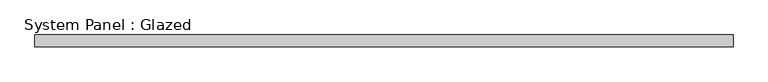
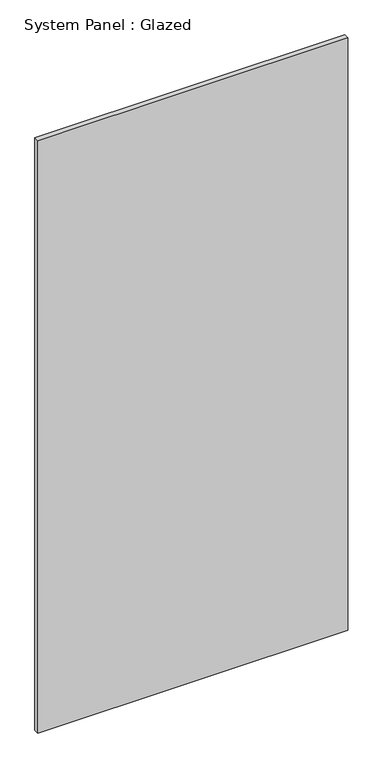
"""IFC4 building model written with IfcOpenShell, lengths in millimetres: plate geometry, System Panel : Glazed."""

from ifc_helpers import new_model, si_unit, origin, origin_with_axes, place, context, project, spatial, polyline, outline, extrude, source, transform, mapped, element, save


def system_panel_glazed_a7f3818b(model_context):
    return source(origin(), model_context, "Body", "SweptSolid", [
        extrude(outline(polyline([(742.475, 24.5), (-742.475, 24.5), (-742.475, 49.5), (742.475, 49.5), (742.475, 24.5)])), origin_with_axes(), (0.0, 0.0, 1.0), 3000.0),
    ])


if __name__ == "__main__":
    model = new_model("IFC4")
    model_context = context("Model", 3, world=origin())
    ifc_project = project(units=[si_unit("LENGTHUNIT", "METRE", prefix="MILLI")], contexts=[model_context])
    site = spatial("IfcSite", under=ifc_project)
    building = spatial("IfcBuilding", under=site)
    placement = place(None, origin())
    system_panel_glazed_shape = system_panel_glazed_a7f3818b(model_context)
    element("IfcPlate", 1, ObjectType="System Panel : Glazed", at=placement, inside=building, context=model_context, shape_type="MappedRepresentation", body=[
        mapped(system_panel_glazed_shape, transform((0.0, 0.0, 0.0), x_axis=(1.0, 0.0, 0.0), y_axis=(0.0, 1.0, 0.0), z_axis=(0.0, 0.0, 1.0))),
    ])
    save(model, "model.ifc")

# Revit data of these elements
# Type "System Panel : Glazed"
#   Keynote = "H11"
#   Construction Type Id = "GSP4R"
#   Analytic Construction = "1/8 in Pilkington single glazing"
#   Visual Light Transmittance = 0.9
#   Solar Heat Gain Coefficient = 0.86
#   Heat Transfer Coefficient (U) = 6.7069 W/(m²·K)
#   Define Thermal Properties by = 1
# Element 1 (IfcPlate, "System Panel : Glazed")
#   Materials on its faces: "Glass"
# Materials
#   "Glass": class "Glass", colour RGB 0 128 192, transparency 0.9, Description = "Soda Lime Glass", Cost = 0
